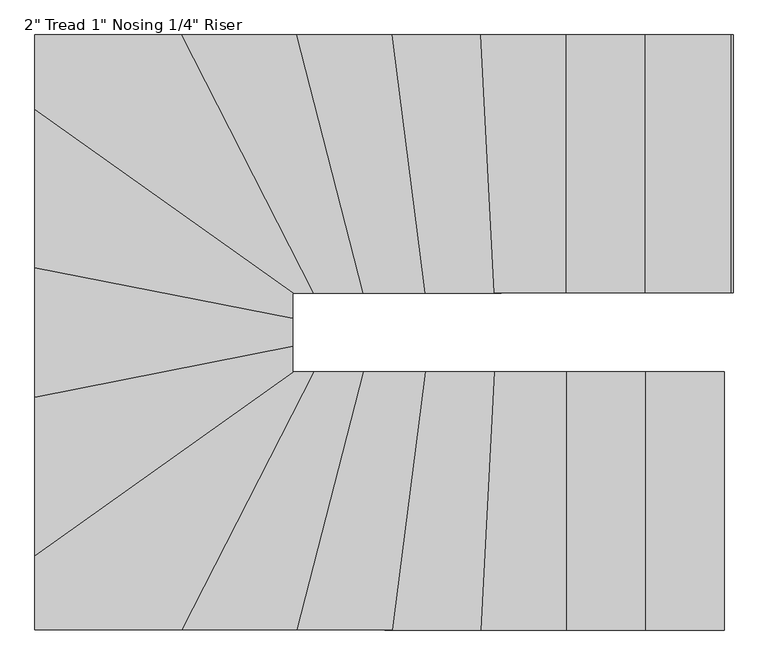
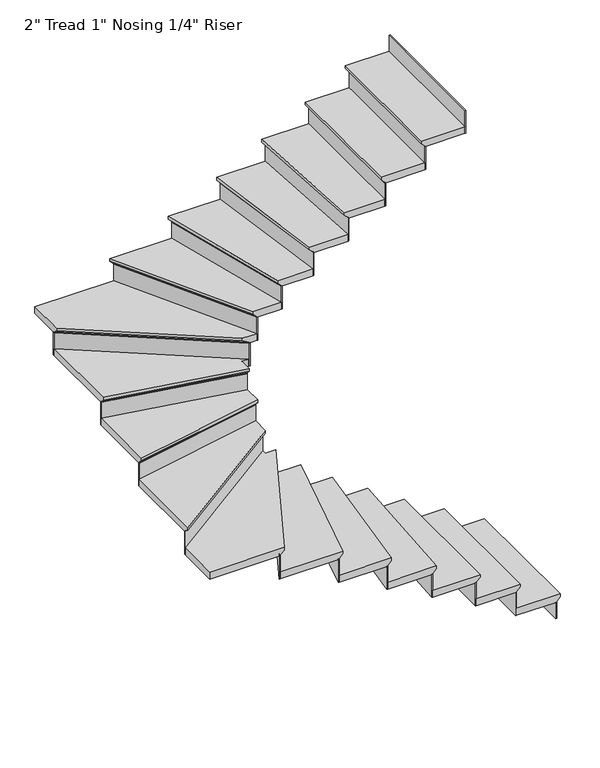
"""IFC4 building model written with IfcOpenShell, lengths in millimetres: stair flight geometry."""

from ifc_helpers import new_model, si_unit, origin, place, context, project, spatial, faceted_brep, source, transform, mapped, element, save


def stair_flight_48a9080d(model_context):
    return source(origin(), model_context, "Body", "Brep", [
        faceted_brep([(-8055.8175858, 298.353629, 150.2833333), (-8055.8175858, 298.353629, 169.3333333), (-8055.8175858, -616.046371, 169.3333333), (-8055.8175858, -616.046371, 150.2833333), (-8081.2175858, 298.353629, 124.8833333), (-8081.2175858, -616.046371, 124.8833333), (-8360.6175858, 298.353629, 169.3333333), (-8360.6175858, -616.046371, 169.3333333), (-8081.2175858, -616.046371, 118.5333333), (-8360.6175858, -616.046371, 118.5333333), (-8360.6175858, 298.353629, 118.5333333), (-8081.2175858, 298.353629, 118.5333333)], [[[0, 1, 2, 3]], [[4, 0, 3, 5]], [[2, 1, 6, 7]], [[8, 9, 10, 11]], [[2, 7, 9, 8, 5, 3]], [[8, 11, 4, 5]], [[6, 1, 0, 4, 11, 10]], [[7, 6, 10, 9]]]),
        faceted_brep([(-8081.2175858, 298.353629, 118.5333333), (-8081.2175858, 298.353629, 0.0), (-8087.5675858, 298.353629, 0.0), (-8087.5675858, 298.353629, 118.5333333), (-8081.2175858, -616.046371, 118.5333333), (-8087.5675858, -616.046371, 118.5333333), (-8087.5675858, -616.046371, 0.0), (-8081.2175858, -616.046371, 0.0)], [[[0, 1, 2, 3]], [[4, 5, 6, 7]], [[1, 0, 4, 7]], [[2, 1, 7, 6]], [[3, 2, 6, 5]], [[0, 3, 5, 4]]]),
        faceted_brep([(-8360.6175858, 298.353629, 287.8666667), (-8360.6175858, 298.353629, 118.5333333), (-8366.9675858, 298.353629, 118.5333333), (-8366.9675858, 298.353629, 287.8666667), (-8360.6175858, -616.046371, 287.8666667), (-8366.9675858, -616.046371, 287.8666667), (-8366.9675858, -616.046371, 118.5333333), (-8360.6175858, -616.046371, 118.5333333)], [[[0, 1, 2, 3]], [[4, 5, 6, 7]], [[1, 0, 4, 7]], [[2, 1, 7, 6]], [[3, 2, 6, 5]], [[0, 3, 5, 4]]]),
        faceted_brep([(-8335.2175858, -616.046371, 338.6666667), (-8335.2175858, 298.353629, 338.6666667), (-8640.0175858, 298.353629, 338.6666667), (-8640.0175858, -616.046371, 338.6666667), (-8360.6175858, -616.046371, 287.8666667), (-8640.0175858, -616.046371, 287.8666667), (-8640.0175858, 298.353629, 287.8666667), (-8360.6175858, 298.353629, 287.8666667), (-8360.6175858, -616.046371, 294.2166667), (-8335.2175858, -616.046371, 319.6166667), (-8360.6175858, 298.353629, 294.2166667), (-8335.2175858, 298.353629, 319.6166667)], [[[0, 1, 2, 3]], [[4, 5, 6, 7]], [[0, 3, 5, 4, 8, 9]], [[4, 7, 10, 8]], [[2, 1, 11, 10, 7, 6]], [[3, 2, 6, 5]], [[11, 1, 0, 9]], [[10, 11, 9, 8]]]),
        faceted_brep([(-8640.0175858, 298.353629, 457.2), (-8640.0175858, 298.353629, 287.8666667), (-8646.3675858, 298.353629, 287.8666667), (-8646.3675858, 298.353629, 457.2), (-8640.0175858, -616.046371, 457.2), (-8646.3675858, -616.046371, 457.2), (-8646.3675858, -616.046371, 287.8666667), (-8640.0175858, -616.046371, 287.8666667)], [[[0, 1, 2, 3]], [[4, 5, 6, 7]], [[1, 0, 4, 7]], [[2, 1, 7, 6]], [[3, 2, 6, 5]], [[0, 3, 5, 4]]]),
        faceted_brep([(-8614.6175858, -616.046371, 508.0), (-8614.6175858, 298.353629, 508.0), (-8895.6847473, 298.353629, 508.0), (-8943.2190177, -616.046371, 508.0), (-8640.0175858, -616.046371, 457.2), (-8943.2190177, -616.046371, 457.2), (-8895.6847473, 298.353629, 457.2), (-8640.0175858, 298.353629, 457.2), (-8640.0175858, -616.046371, 463.55), (-8614.6175858, -616.046371, 488.95), (-8640.0175858, 298.353629, 463.55), (-8614.6175858, 298.353629, 488.95)], [[[0, 1, 2, 3]], [[4, 5, 6, 7]], [[0, 3, 5, 4, 8, 9]], [[4, 7, 10, 8]], [[2, 1, 11, 10, 7, 6]], [[3, 2, 6, 5]], [[11, 1, 0, 9]], [[10, 11, 9, 8]]]),
        faceted_brep([(-8895.6847473, 298.353629, 626.5333333), (-8895.6847473, 298.353629, 457.2), (-8902.0433214, 298.353629, 457.2), (-8902.0433214, 298.353629, 626.5333333), (-8943.2190177, -616.046371, 626.5333333), (-8949.5775918, -616.046371, 626.5333333), (-8949.5775918, -616.046371, 457.2), (-8943.2190177, -616.046371, 457.2)], [[[0, 1, 2, 3]], [[4, 5, 6, 7]], [[1, 0, 4, 7]], [[2, 1, 7, 6]], [[3, 2, 6, 5]], [[0, 3, 5, 4]]]),
        faceted_brep([(-8917.784721, -616.046371, 677.3333333), (-8870.2504506, 298.353629, 677.3333333), (-9139.8514471, 298.353629, 677.3333333), (-9258.2074987, -616.046371, 677.3333333), (-8943.2190177, -616.046371, 626.5333333), (-9258.2074987, -616.046371, 626.5333333), (-9139.8514471, 298.353629, 626.5333333), (-8895.6847473, 298.353629, 626.5333333), (-8943.2190177, -616.046371, 632.8833333), (-8917.784721, -616.046371, 658.2833333), (-8895.6847473, 298.353629, 632.8833333), (-8870.2504506, 298.353629, 658.2833333)], [[[0, 1, 2, 3]], [[4, 5, 6, 7]], [[0, 3, 5, 4, 8, 9]], [[4, 7, 10, 8]], [[2, 1, 11, 10, 7, 6]], [[3, 2, 6, 5]], [[11, 1, 0, 9]], [[10, 11, 9, 8]]]),
        faceted_brep([(-9139.8514471, 298.353629, 795.8666667), (-9139.8514471, 298.353629, 626.5333333), (-9146.2544189, 298.353629, 626.5333333), (-9146.2544189, 298.353629, 795.8666667), (-9258.2074987, -616.046371, 795.8666667), (-9264.6104705, -616.046371, 795.8666667), (-9264.6104705, -616.046371, 626.5333333), (-9258.2074987, -616.046371, 626.5333333)], [[[0, 1, 2, 3]], [[4, 5, 6, 7]], [[1, 0, 4, 7]], [[2, 1, 7, 6]], [[3, 2, 6, 5]], [[0, 3, 5, 4]]]),
        faceted_brep([(-9232.5956116, -616.046371, 846.6666667), (-9114.23956, 298.353629, 846.6666667), (-9361.4786696, 298.353629, 846.6666667), (-9596.609117, -616.046371, 846.6666667), (-9258.2074987, -616.046371, 795.8666667), (-9596.609117, -616.046371, 795.8666667), (-9361.4786696, 298.353629, 795.8666667), (-9139.8514471, 298.353629, 795.8666667), (-9258.2074987, -616.046371, 802.2166667), (-9232.5956116, -616.046371, 827.6166667), (-9139.8514471, 298.353629, 802.2166667), (-9114.23956, 298.353629, 827.6166667)], [[[0, 1, 2, 3]], [[4, 5, 6, 7]], [[0, 3, 5, 4, 8, 9]], [[4, 7, 10, 8]], [[2, 1, 11, 10, 7, 6]], [[3, 2, 6, 5]], [[11, 1, 0, 9]], [[10, 11, 9, 8]]]),
        faceted_brep([(-9361.4786696, 298.353629, 965.2), (-9361.4786696, 298.353629, 795.8666667), (-9368.0352464, 298.353629, 795.8666667), (-9368.0352464, 298.353629, 965.2), (-9596.609117, -616.046371, 965.2), (-9603.1656938, -616.046371, 965.2), (-9603.1656938, -616.046371, 795.8666667), (-9596.609117, -616.046371, 795.8666667)], [[[0, 1, 2, 3]], [[4, 5, 6, 7]], [[1, 0, 4, 7]], [[2, 1, 7, 6]], [[3, 2, 6, 5]], [[0, 3, 5, 4]]]),
        faceted_brep([(-9570.3828095, -616.046371, 1016.0), (-9335.2523621, 298.353629, 1016.0), (-9537.8253056, 298.353629, 1016.0), (-10006.649927, -616.046371, 1016.0), (-9596.609117, -616.046371, 965.2), (-10006.649927, -616.046371, 965.2), (-9537.8253056, 298.353629, 965.2), (-9361.4786696, 298.353629, 965.2), (-9596.609117, -616.046371, 971.55), (-9570.3828095, -616.046371, 996.95), (-9361.4786696, 298.353629, 971.55), (-9335.2523621, 298.353629, 996.95)], [[[0, 1, 2, 3]], [[4, 5, 6, 7]], [[0, 3, 5, 4, 8, 9]], [[4, 7, 10, 8]], [[2, 1, 11, 10, 7, 6]], [[3, 2, 6, 5]], [[11, 1, 0, 9]], [[10, 11, 9, 8]]]),
        faceted_brep([(-9537.8253056, 298.353629, 1134.5333333), (-9537.8253056, 298.353629, 965.2), (-9544.9612888, 298.353629, 965.2), (-9544.9612888, 298.353629, 1134.5333333), (-10006.649927, -616.046371, 1134.5333333), (-10013.7859101, -616.046371, 1134.5333333), (-10013.7859101, -616.046371, 965.2), (-10006.649927, -616.046371, 965.2)], [[[0, 1, 2, 3]], [[4, 5, 6, 7]], [[1, 0, 4, 7]], [[2, 1, 7, 6]], [[3, 2, 6, 5]], [[0, 3, 5, 4]]]),
        faceted_brep([(-10497.9492777, -322.3652373, 1185.3333333), (-10497.9492777, -616.046371, 1185.3333333), (-9978.1059944, -616.046371, 1185.3333333), (-9509.2813731, 298.353629, 1185.3333333), (-9583.5492777, 298.353629, 1185.3333333), (-9583.5492777, 327.9087119, 1185.3333333), (-10497.9492777, -616.046371, 1134.5333333), (-10497.9492777, -322.3652373, 1134.5333333), (-9583.5492777, 327.9087119, 1134.5333333), (-9583.5492777, 298.353629, 1134.5333333), (-9537.8253056, 298.353629, 1134.5333333), (-10006.649927, -616.046371, 1134.5333333), (-10006.649927, -616.046371, 1140.8833333), (-9978.1059944, -616.046371, 1166.2833333), (-9537.8253056, 298.353629, 1140.8833333), (-9509.2813731, 298.353629, 1166.2833333)], [[[0, 1, 2, 3, 4, 5]], [[6, 7, 8, 9, 10, 11]], [[1, 0, 7, 6]], [[2, 1, 6, 11, 12, 13]], [[11, 10, 14, 12]], [[4, 3, 15, 14, 10, 9]], [[5, 4, 9, 8]], [[0, 5, 8, 7]], [[15, 3, 2, 13]], [[14, 15, 13, 12]]]),
        faceted_brep([(-9583.5492777, 327.9087119, 1303.8666667), (-9583.5492777, 327.9087119, 1134.5333333), (-9583.5492777, 335.7006867, 1134.5333333), (-9583.5492777, 335.7006867, 1303.8666667), (-10497.9492777, -322.3652373, 1303.8666667), (-10497.9492777, -314.5732625, 1303.8666667), (-10497.9492777, -314.5732625, 1134.5333333), (-10497.9492777, -322.3652373, 1134.5333333)], [[[0, 1, 2, 3]], [[4, 5, 6, 7]], [[1, 0, 4, 7]], [[2, 1, 7, 6]], [[3, 2, 6, 5]], [[0, 3, 5, 4]]]),
        faceted_brep([(-10497.9492777, -353.5331365, 1354.6666667), (-9583.5492777, 296.7408127, 1354.6666667), (-9583.5492777, 414.3627989, 1354.6666667), (-10497.9492777, 234.1219426, 1354.6666667), (-10497.9492777, -322.3652373, 1303.8666667), (-10497.9492777, 234.1219426, 1303.8666667), (-9583.5492777, 414.3627989, 1303.8666667), (-9583.5492777, 327.9087119, 1303.8666667), (-10497.9492777, -322.3652373, 1310.2166667), (-10497.9492777, -353.5331365, 1335.6166667), (-9583.5492777, 327.9087119, 1310.2166667), (-9583.5492777, 296.7408127, 1335.6166667)], [[[0, 1, 2, 3]], [[4, 5, 6, 7]], [[0, 3, 5, 4, 8, 9]], [[4, 7, 10, 8]], [[2, 1, 11, 10, 7, 6]], [[3, 2, 6, 5]], [[11, 1, 0, 9]], [[10, 11, 9, 8]]]),
        faceted_brep([(-9583.5492777, 414.3627989, 1473.2), (-9583.5492777, 414.3627989, 1303.8666667), (-9583.5492777, 420.8349844, 1303.8666667), (-9583.5492777, 420.8349844, 1473.2), (-10497.9492777, 234.1219426, 1473.2), (-10497.9492777, 240.594128, 1473.2), (-10497.9492777, 240.594128, 1303.8666667), (-10497.9492777, 234.1219426, 1303.8666667)], [[[0, 1, 2, 3]], [[4, 5, 6, 7]], [[1, 0, 4, 7]], [[2, 1, 7, 6]], [[3, 2, 6, 5]], [[0, 3, 5, 4]]]),
        faceted_brep([(-10497.9492777, 208.2332009, 1524.0), (-9583.5492777, 388.4740572, 1524.0), (-9583.5492777, 513.5219426, 1524.0), (-10497.9492777, 693.7627989, 1524.0), (-10497.9492777, 234.1219426, 1473.2), (-10497.9492777, 693.7627989, 1473.2), (-9583.5492777, 513.5219426, 1473.2), (-9583.5492777, 414.3627989, 1473.2), (-10497.9492777, 234.1219426, 1479.55), (-10497.9492777, 208.2332009, 1504.95), (-9583.5492777, 414.3627989, 1479.55), (-9583.5492777, 388.4740572, 1504.95)], [[[0, 1, 2, 3]], [[4, 5, 6, 7]], [[0, 3, 5, 4, 8, 9]], [[4, 7, 10, 8]], [[2, 1, 11, 10, 7, 6]], [[3, 2, 6, 5]], [[11, 1, 0, 9]], [[10, 11, 9, 8]]]),
        faceted_brep([(-9583.5492777, 513.5219426, 1642.5333333), (-9583.5492777, 513.5219426, 1473.2), (-9583.5492777, 519.994128, 1473.2), (-9583.5492777, 519.994128, 1642.5333333), (-10497.9492777, 693.7627989, 1642.5333333), (-10497.9492777, 700.2349844, 1642.5333333), (-10497.9492777, 700.2349844, 1473.2), (-10497.9492777, 693.7627989, 1473.2)], [[[0, 1, 2, 3]], [[4, 5, 6, 7]], [[1, 0, 4, 7]], [[2, 1, 7, 6]], [[3, 2, 6, 5]], [[0, 3, 5, 4]]]),
        faceted_brep([(-10497.9492777, 667.8740572, 1693.3333333), (-9583.5492777, 487.6332009, 1693.3333333), (-9583.5492777, 577.753629, 1693.3333333), (-9537.4538031, 577.753629, 1693.3333333), (-10497.9492777, 1260.8082937, 1693.3333333), (-10497.9492777, 693.7627989, 1642.5333333), (-10497.9492777, 1260.8082937, 1642.5333333), (-9537.4538031, 577.753629, 1642.5333333), (-9583.5492777, 577.753629, 1642.5333333), (-9583.5492777, 513.5219426, 1642.5333333), (-10497.9492777, 693.7627989, 1648.8833333), (-10497.9492777, 667.8740572, 1674.2833333), (-9583.5492777, 513.5219426, 1648.8833333), (-9583.5492777, 487.6332009, 1674.2833333)], [[[0, 1, 2, 3, 4]], [[5, 6, 7, 8, 9]], [[0, 4, 6, 5, 10, 11]], [[5, 9, 12, 10]], [[2, 1, 13, 12, 9, 8]], [[3, 2, 8, 7]], [[4, 3, 7, 6]], [[13, 1, 0, 11]], [[12, 13, 11, 10]]]),
        faceted_brep([(-9537.4538031, 577.753629, 1811.8666667), (-9537.4538031, 577.753629, 1642.5333333), (-9526.4969106, 577.753629, 1642.5333333), (-9526.4969106, 577.753629, 1811.8666667), (-10497.9492777, 1260.8082937, 1811.8666667), (-10497.9492777, 1268.6002685, 1811.8666667), (-10497.9492777, 1268.6002685, 1642.5333333), (-10497.9492777, 1260.8082937, 1642.5333333)], [[[0, 1, 2, 3]], [[4, 5, 6, 7]], [[1, 0, 4, 7]], [[2, 1, 7, 6]], [[3, 2, 6, 5]], [[0, 3, 5, 4]]]),
        faceted_brep([(-9949.5620619, 1492.153629, 1862.6666667), (-10497.9492777, 1492.153629, 1862.6666667), (-10497.9492777, 1229.6403945, 1862.6666667), (-9581.2813731, 577.753629, 1862.6666667), (-9480.7374406, 577.753629, 1862.6666667), (-10497.9492777, 1492.153629, 1811.8666667), (-9949.5620619, 1492.153629, 1811.8666667), (-9480.7374406, 577.753629, 1811.8666667), (-9537.4538031, 577.753629, 1811.8666667), (-10497.9492777, 1260.8082937, 1811.8666667), (-10497.9492777, 1260.8082937, 1818.2166667), (-10497.9492777, 1229.6403945, 1843.6166667), (-9537.4538031, 577.753629, 1818.2166667), (-9581.2813731, 577.753629, 1843.6166667)], [[[0, 1, 2, 3, 4]], [[5, 6, 7, 8, 9]], [[1, 0, 6, 5]], [[2, 1, 5, 9, 10, 11]], [[9, 8, 12, 10]], [[4, 3, 13, 12, 8, 7]], [[0, 4, 7, 6]], [[13, 3, 2, 11]], [[12, 13, 11, 10]]]),
        faceted_brep([(-9480.7374406, 577.753629, 1981.2), (-9480.7374406, 577.753629, 1811.8666667), (-9473.6014574, 577.753629, 1811.8666667), (-9473.6014574, 577.753629, 1981.2), (-9949.5620619, 1492.153629, 1981.2), (-9942.4260788, 1492.153629, 1981.2), (-9942.4260788, 1492.153629, 1811.8666667), (-9949.5620619, 1492.153629, 1811.8666667)], [[[0, 1, 2, 3]], [[4, 5, 6, 7]], [[1, 0, 4, 7]], [[2, 1, 7, 6]], [[3, 2, 6, 5]], [[0, 3, 5, 4]]]),
        faceted_brep([(-9978.1059944, 1492.153629, 2032.0), (-9509.2813731, 577.753629, 2032.0), (-9309.0260546, 577.753629, 2032.0), (-9544.156502, 1492.153629, 2032.0), (-9949.5620619, 1492.153629, 1981.2), (-9544.156502, 1492.153629, 1981.2), (-9309.0260546, 577.753629, 1981.2), (-9480.7374406, 577.753629, 1981.2), (-9949.5620619, 1492.153629, 1987.55), (-9978.1059944, 1492.153629, 2012.95), (-9480.7374406, 577.753629, 1987.55), (-9509.2813731, 577.753629, 2012.95)], [[[0, 1, 2, 3]], [[4, 5, 6, 7]], [[0, 3, 5, 4, 8, 9]], [[4, 7, 10, 8]], [[2, 1, 11, 10, 7, 6]], [[3, 2, 6, 5]], [[11, 1, 0, 9]], [[10, 11, 9, 8]]]),
        faceted_brep([(-9309.0260546, 577.753629, 2150.5333333), (-9309.0260546, 577.753629, 1981.2), (-9302.4694778, 577.753629, 1981.2), (-9302.4694778, 577.753629, 2150.5333333), (-9544.156502, 1492.153629, 2150.5333333), (-9537.5999252, 1492.153629, 2150.5333333), (-9537.5999252, 1492.153629, 1981.2), (-9544.156502, 1492.153629, 1981.2)], [[[0, 1, 2, 3]], [[4, 5, 6, 7]], [[1, 0, 4, 7]], [[2, 1, 7, 6]], [[3, 2, 6, 5]], [[0, 3, 5, 4]]]),
        faceted_brep([(-9570.3828095, 1492.153629, 2201.3333333), (-9335.2523621, 577.753629, 2201.3333333), (-9088.6276729, 577.753629, 2201.3333333), (-9206.9837245, 1492.153629, 2201.3333333), (-9544.156502, 1492.153629, 2150.5333333), (-9206.9837245, 1492.153629, 2150.5333333), (-9088.6276729, 577.753629, 2150.5333333), (-9309.0260546, 577.753629, 2150.5333333), (-9544.156502, 1492.153629, 2156.8833333), (-9570.3828095, 1492.153629, 2182.2833333), (-9309.0260546, 577.753629, 2156.8833333), (-9335.2523621, 577.753629, 2182.2833333)], [[[0, 1, 2, 3]], [[4, 5, 6, 7]], [[0, 3, 5, 4, 8, 9]], [[4, 7, 10, 8]], [[2, 1, 11, 10, 7, 6]], [[3, 2, 6, 5]], [[11, 1, 0, 9]], [[10, 11, 9, 8]]]),
        faceted_brep([(-9088.6276729, 577.753629, 2319.8666667), (-9088.6276729, 577.753629, 2150.5333333), (-9082.2247011, 577.753629, 2150.5333333), (-9082.2247011, 577.753629, 2319.8666667), (-9206.9837245, 1492.153629, 2319.8666667), (-9200.5807527, 1492.153629, 2319.8666667), (-9200.5807527, 1492.153629, 2150.5333333), (-9206.9837245, 1492.153629, 2150.5333333)], [[[0, 1, 2, 3]], [[4, 5, 6, 7]], [[1, 0, 4, 7]], [[2, 1, 7, 6]], [[3, 2, 6, 5]], [[0, 3, 5, 4]]]),
        faceted_brep([(-9232.5956116, 1492.153629, 2370.6666667), (-9114.23956, 577.753629, 2370.6666667), (-8844.8161539, 577.753629, 2370.6666667), (-8892.3504243, 1492.153629, 2370.6666667), (-9206.9837245, 1492.153629, 2319.8666667), (-8892.3504243, 1492.153629, 2319.8666667), (-8844.8161539, 577.753629, 2319.8666667), (-9088.6276729, 577.753629, 2319.8666667), (-9206.9837245, 1492.153629, 2326.2166667), (-9232.5956116, 1492.153629, 2351.6166667), (-9088.6276729, 577.753629, 2326.2166667), (-9114.23956, 577.753629, 2351.6166667)], [[[0, 1, 2, 3]], [[4, 5, 6, 7]], [[0, 3, 5, 4, 8, 9]], [[4, 7, 10, 8]], [[2, 1, 11, 10, 7, 6]], [[3, 2, 6, 5]], [[11, 1, 0, 9]], [[10, 11, 9, 8]]]),
        faceted_brep([(-8844.8161539, 577.753629, 2489.2), (-8844.8161539, 577.753629, 2319.8666667), (-8838.4575798, 577.753629, 2319.8666667), (-8838.4575798, 577.753629, 2489.2), (-8892.3504243, 1492.153629, 2489.2), (-8885.9918502, 1492.153629, 2489.2), (-8885.9918502, 1492.153629, 2319.8666667), (-8892.3504243, 1492.153629, 2319.8666667)], [[[0, 1, 2, 3]], [[4, 5, 6, 7]], [[1, 0, 4, 7]], [[2, 1, 7, 6]], [[3, 2, 6, 5]], [[0, 3, 5, 4]]]),
        faceted_brep([(-8917.784721, 1492.153629, 2540.0), (-8870.2504506, 577.753629, 2540.0), (-8589.2175858, 577.753629, 2540.0), (-8589.2175858, 1492.153629, 2540.0), (-8892.3504243, 1492.153629, 2489.2), (-8589.2175858, 1492.153629, 2489.2), (-8589.2175858, 577.753629, 2489.2), (-8844.8161539, 577.753629, 2489.2), (-8892.3504243, 1492.153629, 2495.55), (-8917.784721, 1492.153629, 2520.95), (-8844.8161539, 577.753629, 2495.55), (-8870.2504506, 577.753629, 2520.95)], [[[0, 1, 2, 3]], [[4, 5, 6, 7]], [[0, 3, 5, 4, 8, 9]], [[4, 7, 10, 8]], [[2, 1, 11, 10, 7, 6]], [[3, 2, 6, 5]], [[11, 1, 0, 9]], [[10, 11, 9, 8]]]),
        faceted_brep([(-8589.2175858, 577.753629, 2658.5333333), (-8589.2175858, 577.753629, 2489.2), (-8582.8675858, 577.753629, 2489.2), (-8582.8675858, 577.753629, 2658.5333333), (-8589.2175858, 1492.153629, 2658.5333333), (-8582.8675858, 1492.153629, 2658.5333333), (-8582.8675858, 1492.153629, 2489.2), (-8589.2175858, 1492.153629, 2489.2)], [[[0, 1, 2, 3]], [[4, 5, 6, 7]], [[1, 0, 4, 7]], [[2, 1, 7, 6]], [[3, 2, 6, 5]], [[0, 3, 5, 4]]]),
        faceted_brep([(-8614.6175858, 1492.153629, 2709.3333333), (-8614.6175858, 577.753629, 2709.3333333), (-8309.8175858, 577.753629, 2709.3333333), (-8309.8175858, 1492.153629, 2709.3333333), (-8589.2175858, 1492.153629, 2658.5333333), (-8309.8175858, 1492.153629, 2658.5333333), (-8309.8175858, 577.753629, 2658.5333333), (-8589.2175858, 577.753629, 2658.5333333), (-8589.2175858, 1492.153629, 2664.8833333), (-8614.6175858, 1492.153629, 2690.2833333), (-8589.2175858, 577.753629, 2664.8833333), (-8614.6175858, 577.753629, 2690.2833333)], [[[0, 1, 2, 3]], [[4, 5, 6, 7]], [[0, 3, 5, 4, 8, 9]], [[4, 7, 10, 8]], [[2, 1, 11, 10, 7, 6]], [[3, 2, 6, 5]], [[11, 1, 0, 9]], [[10, 11, 9, 8]]]),
        faceted_brep([(-8309.8175858, 577.753629, 2827.8666667), (-8309.8175858, 577.753629, 2658.5333333), (-8303.4675858, 577.753629, 2658.5333333), (-8303.4675858, 577.753629, 2827.8666667), (-8309.8175858, 1492.153629, 2827.8666667), (-8303.4675858, 1492.153629, 2827.8666667), (-8303.4675858, 1492.153629, 2658.5333333), (-8309.8175858, 1492.153629, 2658.5333333)], [[[0, 1, 2, 3]], [[4, 5, 6, 7]], [[1, 0, 4, 7]], [[2, 1, 7, 6]], [[3, 2, 6, 5]], [[0, 3, 5, 4]]]),
        faceted_brep([(-8030.4175858, 577.753629, 2997.2), (-8030.4175858, 577.753629, 2827.8666667), (-8024.0675858, 577.753629, 2827.8666667), (-8024.0675858, 577.753629, 2997.2), (-8030.4175858, 1492.153629, 2997.2), (-8024.0675858, 1492.153629, 2997.2), (-8024.0675858, 1492.153629, 2827.8666667), (-8030.4175858, 1492.153629, 2827.8666667)], [[[0, 1, 2, 3]], [[4, 5, 6, 7]], [[1, 0, 4, 7]], [[2, 1, 7, 6]], [[3, 2, 6, 5]], [[0, 3, 5, 4]]]),
        faceted_brep([(-8335.2175858, 1492.153629, 2878.6666667), (-8335.2175858, 577.753629, 2878.6666667), (-8030.4175858, 577.753629, 2878.6666667), (-8030.4175858, 1492.153629, 2878.6666667), (-8309.8175858, 1492.153629, 2827.8666667), (-8030.4175858, 1492.153629, 2827.8666667), (-8030.4175858, 577.753629, 2827.8666667), (-8309.8175858, 577.753629, 2827.8666667), (-8309.8175858, 1492.153629, 2834.2166667), (-8335.2175858, 1492.153629, 2859.6166667), (-8309.8175858, 577.753629, 2834.2166667), (-8335.2175858, 577.753629, 2859.6166667)], [[[0, 1, 2, 3]], [[4, 5, 6, 7]], [[0, 3, 5, 4, 8, 9]], [[4, 7, 10, 8]], [[2, 1, 11, 10, 7, 6]], [[3, 2, 6, 5]], [[11, 1, 0, 9]], [[10, 11, 9, 8]]]),
    ])


if __name__ == "__main__":
    model = new_model("IFC4")
    model_context = context("Model", 3, world=origin())
    ifc_project = project(units=[si_unit("LENGTHUNIT", "METRE", prefix="MILLI")], contexts=[model_context])
    site = spatial("IfcSite", under=ifc_project)
    building = spatial("IfcBuilding", under=site)
    placement = place(None, origin())
    stair_flight_shape = stair_flight_48a9080d(model_context)
    element("IfcStairFlight", 1, ObjectType="2\" Tread 1\" Nosing 1/4\" Riser", at=placement, inside=building, context=model_context, shape_type="MappedRepresentation", body=[
        mapped(stair_flight_shape, transform((0.0, 0.0, 0.0), x_axis=(1.0, 0.0, 0.0), y_axis=(0.0, 1.0, 0.0), z_axis=(0.0, 0.0, 1.0))),
    ])
    save(model, "model.ifc")
